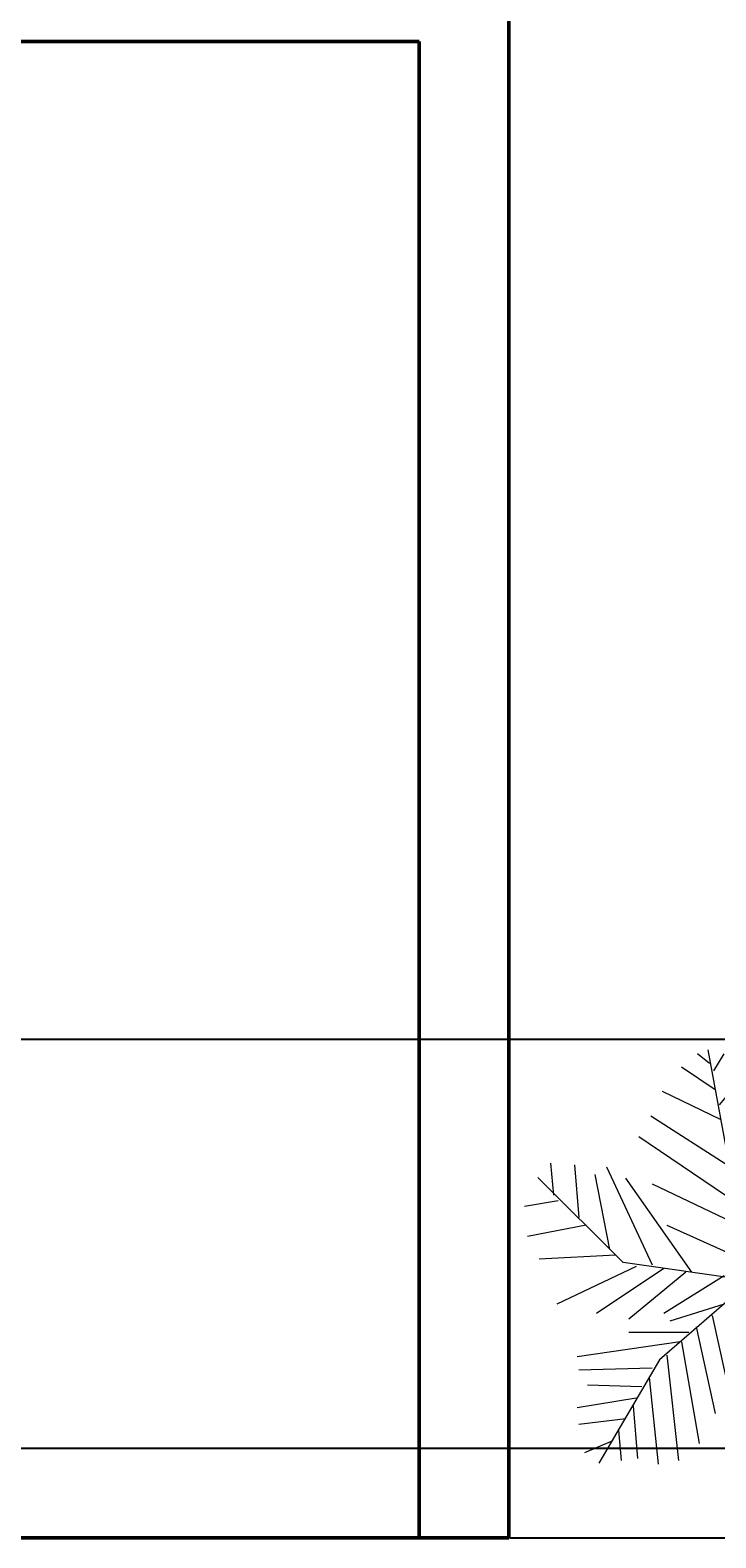
# Model space of a CAD drawing. Units: inches. Extents: x 37 to 824, y -700 to 234.
# Tile 38 of 77: x 380 to 449, y -366 to -215. Entities that reach past the tile are written whole.
import ezdxf

# ---------------------------------------------------------------- set-up
doc = ezdxf.new("R2010")
doc.units = ezdxf.units.IN
doc.header["$MEASUREMENT"] = 0
for name, color, linetype, lineweight in [('A-ANNO-DIMS', 2, 'Continuous', 18), ('A-SITE-PLNT', 3, 'Continuous', 13), ('A-WALL', 2, 'Continuous', 50)]:
    doc.layers.add(name, color=color, linetype=linetype, lineweight=lineweight)
doc.styles.get("Standard").update_dxf_attribs({"font": 'arial.ttf'})
doc.dimstyles.get("Standard").update_dxf_attribs({"dimtxt": 0.18, "dimasz": 0.18, "dimexe": 0.18, "dimexo": 0.0625, "dimgap": 0.09, "dimtad": 0, "dimtih": 1, "dimtoh": 1, "dimdec": 1, "dimzin": 0, "dimdsep": 46, "dimlunit": 4, "dimtxsty": 'Standard', "dimcen": 0.09, "dimadec": 0, "dimazin": 0, "dimtfac": 1, "dimtdec": 1, "dimtofl": 0, "dimtmove": 0, "dimatfit": 3, "dimfxl": 1, "dimtolj": 1, "dimtzin": 0, "dimarcsym": 0})

# ---------------------------------------------------------------- blocks, each defined once
blk = doc.blocks.new('*U33')
for p, q in [((-10.186, 53.64), (-13.084, 55.962)), ((0, 0), (-10.5, 57)), ((-9.099, 51.782), (-6.563, 55.962)), ((-8.737, 47.138), (-17.069, 52.711)), ((-7.65, 43.423), (-2.578, 49.46)), ((-7.288, 39.707), (-21.778, 46.673)), ((-5.839, 35.992), (4.667, 48.067)), ((-5.114, 27.632), (10.463, 46.673)), ((-5.114, 28.097), (-24.676, 40.636)), ((-2.941, 16.486), (8.652, 37.85)), ((-3.665, 19.273), (-27.574, 35.527)), ((27, 9), (48, 36)), ((27.127, 9.056), (31.112, 35.992)), ((38.719, 34.134), (41.979, 28.561)), ((44.153, 36.456), (45.239, 32.741)), ((16.259, 5.805), (23.142, 31.348)), ((22.055, 7.198), (27.489, 32.277)), ((31.836, 30.883), (32.561, 16.486)), ((35.096, 32.741), (37.27, 22.524)), ((43.791, 29.954), (51.036, 30.883)), ((-48.585, 21.131), (-49.309, 29.026)), ((-43.513, 28.561), (-42.427, 15.558)), ((-38.442, 26.239), (-34.819, 7.663)), ((-35.544, 28.097), (-24.314, 3.947)), ((-1.129, 6.734), (9.014, 26.704)), ((10.101, 3.483), (17.708, 26.239)), ((-31.5, 4.5), (-52.5, 25.5)), ((-14.533, 2.09), (-30.834, 25.31)), ((-24.314, 23.917), (-2.941, 13.7)), ((3.942, 1.625), (11.187, 24.381)), ((40.53, 25.775), (48.862, 24.846)), ((-47.498, 19.737), (-55.83, 18.344)), ((36.183, 19.737), (48.137, 17.88)), ((33.285, 16.486), (48.862, 10.913)), ((-40.615, 13.7), (-55.105, 10.913)), ((-20.691, 13.7), (-1.129, 4.876)), ((29.662, 12.307), (48.137, 6.269)), ((0, 0), (27, 9)), ((24.229, 7.663), (46.688, 1.625)), ((-33.37, 6.269), (-52.207, 5.34)), ((0, 0), (-31.5, 4.5)), ((18.07, 5.805), (35.096, -3.483)), ((-28.299, 3.483), (-47.86, -5.805)), ((-21.416, 3.018), (-38.079, -8.128)), ((-15.982, 2.09), (-30.11, -9.521)), ((0, 0), (-22.5, -19.5)), ((-6.563, 1.161), (-21.416, -8.128)), ((0, 0), (18, -22.5)), ((6.478, 1.625), (26.04, -8.592)), ((11.187, 3.483), (30.749, -5.805)), ((-4.752, -3.483), (-3.665, -14.629)), ((2.493, -3.019), (-1.491, -20.202)), ((1.769, -2.555), (24.229, -9.521)), ((-6.563, -5.805), (-19.967, -9.985)), ((5.029, -6.27), (2.131, -25.775)), ((-9.461, -8.592), (-6.201, -23.453)), ((7.565, -9.056), (32.198, -14.629)), ((-15.257, -12.772), (-30.11, -12.772)), ((-13.446, -11.378), (-8.737, -32.741)), ((9.014, -11.378), (3.58, -35.992)), ((-17.431, -15.094), (-42.789, -18.809)), ((-20.691, -18.345), (-17.793, -44.352)), ((-17.069, -15.094), (-12.721, -40.172)), ((14.085, -16.951), (6.478, -40.172)), ((12.274, -15.094), (36.907, -18.809)), ((-24.314, -21.596), (-42.427, -22.06)), ((-22.5, -19.5), (-37.5, -45)), ((16.259, -19.738), (36.183, -22.989)), ((-26.849, -26.24), (-40.253, -25.775)), ((-25.038, -23.918), (-22.865, -45.281)), ((18.07, -22.524), (8.289, -45.745)), ((18, -22.5), (27, -52.5)), ((18.433, -22.524), (40.53, -29.026)), ((19.157, -25.311), (38.719, -33.206)), ((-28.299, -29.026), (-42.789, -31.348)), ((-29.023, -30.884), (-27.936, -43.887)), ((20.244, -30.419), (15.897, -44.816)), ((21.331, -32.741), (39.081, -40.636)), ((-30.834, -34.135), (-42.427, -35.528)), ((-32.646, -36.921), (-31.921, -44.352)), ((-34.457, -39.708), (-40.978, -42.494)), ((22.78, -37.85), (19.519, -48.532)), ((22.78, -38.314), (34.372, -44.816)), ((24.591, -43.423), (30.749, -47.603)), ((24.591, -45.745), (23.142, -50.854)), ((26.764, -49.925), (28.213, -50.854))]:
    blk.add_line(p, q)
blk = doc.blocks.new('*D64')
at = {"layer": 'A-ANNO-DIMS', "color": 0, "lineweight": -2, "ltscale": 0.5, "transparency": 16777216}
for p, q in [((428.14, 191.09), (513.77, 191.09)), ((513.59, 190.91), (513.59, -87.23)), ((513.59, -365.73), (513.59, -87.59)), ((428.14, -365.91), (513.77, -365.91))]:
    blk.add_line(p, q, dxfattribs=at)
at = {"layer": 'A-ANNO-DIMS', "color": 0, "ltscale": 0.5, "transparency": 16777216}
for points in [[(513.56, 190.91), (513.62, 190.91), (513.59, 191.09)], [(513.56, -365.73), (513.62, -365.73), (513.59, -365.91)]]:
    blk.add_solid(points, dxfattribs=at)
at = {"layer": 'Defpoints', "color": 0, "ltscale": 0.5, "transparency": 16777216}
for p in [(428.08, 191.09), (428.08, -365.91), (513.59, -365.91)]:
    blk.add_point(p, dxfattribs=at)
at = {"layer": 'A-ANNO-DIMS', "color": 0, "ltscale": 0.5, "transparency": 16777216, "insert": (513.59, -87.41), "char_height": 0.18, "attachment_point": 5}
blk.add_mtext('\\A1;46\'-5"', dxfattribs=at)
blk = doc.blocks.new('*D65')
at = {"layer": 'A-ANNO-DIMS', "color": 0, "lineweight": -2, "ltscale": 0.5, "transparency": 16777216}
for p, q in [((428.14, -178.91), (513.77, -178.91)), ((513.59, -179.09), (513.59, -272.23)), ((513.59, -365.73), (513.59, -272.59)), ((428.14, -365.91), (513.77, -365.91))]:
    blk.add_line(p, q, dxfattribs=at)
at = {"layer": 'A-ANNO-DIMS', "color": 0, "ltscale": 0.5, "transparency": 16777216}
for points in [[(513.56, -179.09), (513.62, -179.09), (513.59, -178.91)], [(513.56, -365.73), (513.62, -365.73), (513.59, -365.91)]]:
    blk.add_solid(points, dxfattribs=at)
at = {"layer": 'Defpoints', "color": 0, "ltscale": 0.5, "transparency": 16777216}
for p in [(428.08, -178.91), (428.08, -365.91), (513.59, -365.91)]:
    blk.add_point(p, dxfattribs=at)
at = {"layer": 'A-ANNO-DIMS', "color": 0, "ltscale": 0.5, "transparency": 16777216, "insert": (513.59, -272.41), "char_height": 0.18, "attachment_point": 5}
blk.add_mtext('\\A1;15\'-7"', dxfattribs=at)
blk = doc.blocks.new('*D88')
at = {"layer": 'A-ANNO-DIMS', "color": 0, "lineweight": -2, "ltscale": 0.5, "transparency": 16777216}
for p, q in [((296.14, -315.91), (513.77, -315.91)), ((513.59, -316.09), (513.59, -336.23)), ((513.59, -356.73), (513.59, -336.59)), ((296.14, -356.91), (513.77, -356.91))]:
    blk.add_line(p, q, dxfattribs=at)
at = {"layer": 'A-ANNO-DIMS', "color": 0, "ltscale": 0.5, "transparency": 16777216}
for points in [[(513.56, -316.09), (513.62, -316.09), (513.59, -315.91)], [(513.56, -356.73), (513.62, -356.73), (513.59, -356.91)]]:
    blk.add_solid(points, dxfattribs=at)
at = {"layer": 'Defpoints', "color": 0, "ltscale": 0.5, "transparency": 16777216}
for p in [(296.08, -315.91), (296.08, -356.91), (513.59, -356.91)]:
    blk.add_point(p, dxfattribs=at)
at = {"layer": 'A-ANNO-DIMS', "color": 0, "ltscale": 0.5, "transparency": 16777216, "insert": (513.59, -336.41), "char_height": 0.18, "attachment_point": 5}
blk.add_mtext('\\A1;3\'-5"', dxfattribs=at)

msp = doc.modelspace()

# ---------------------------------------------------------------- linework, layer by layer
at = {"layer": 'A-WALL'}
for p, q in [((428.08, -110.91), (428.08, -215.91)), ((419.08, -215.91), (358.13, -215.91)), ((419.08, -215.91), (419.08, -365.91)), ((428.08, -215.91), (428.08, -365.91)), ((428.08, -365.91), (161.08, -365.91))]:
    msp.add_line(p, q, dxfattribs=at)

# ---------------------------------------------------------------- block references
at = {"layer": 'A-SITE-PLNT', "xscale": 0.406169560041474, "yscale": 0.406169560041474, "zscale": 0.406169560041474}
msp.add_blockref('*U33', (452.33, -340.13), dxfattribs=at)

# ---------------------------------------------------------------- dimensions: what is measured, and where the dimension line sits
at = {"layer": 'A-ANNO-DIMS', "ltscale": 0.5}
for base, p1, p2, picture, middle in [((513.59, -365.91), (428.08, 191.09), (428.08, -365.91), '*D64', (513.59, -87.41)), ((513.59, -365.91), (428.08, -178.91), (428.08, -365.91), '*D65', (513.59, -272.41)), ((513.59, -356.91), (296.08, -315.91), (296.08, -356.91), '*D88', (513.59, -336.41))]:
    dim = msp.add_linear_dim(base=base, p1=p1, p2=p2, angle=90, dimstyle='Standard', override={"dimdec": 1, "dimlfac": 1, "dimrnd": 0, "dimzin": 1, "dimdsep": 46, "dimlunit": 4, "dimfrac": 2}, dxfattribs=at)
    dim.commit()
    dim.dimension.update_dxf_attribs({"geometry": picture, "text_midpoint": middle})

doc.saveas('drawing.dxf')
